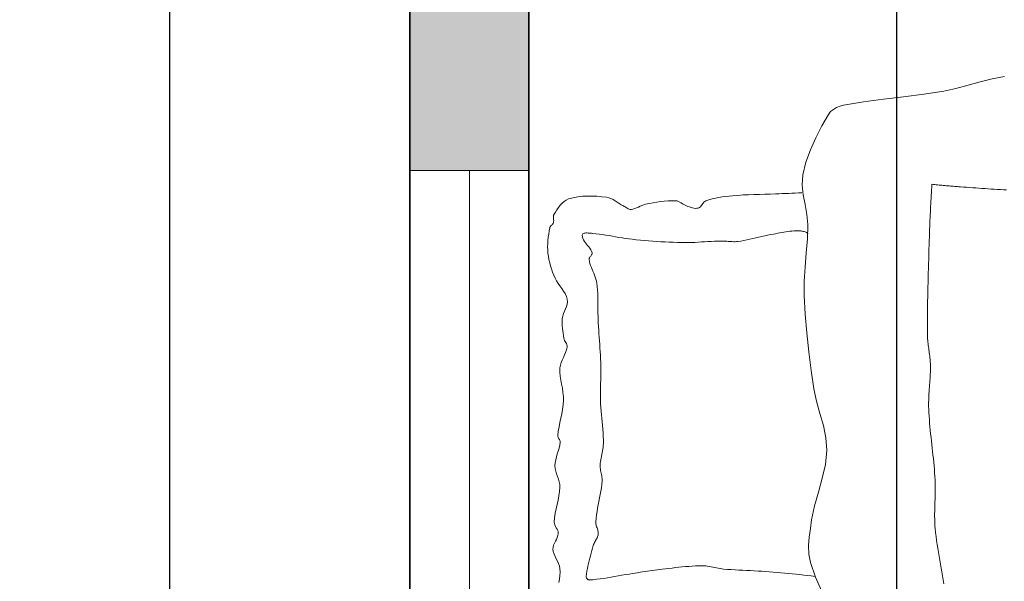
# Model space of a CAD drawing. Units: inches. Extents: x -15 to 423, y -713 to 71.
# Tile 7 of 24: x -4 to 70, y -159 to -117. Entities that reach past the tile are written whole.
import ezdxf

# ---------------------------------------------------------------- set-up
doc = ezdxf.new("R2010")
doc.units = ezdxf.units.IN
doc.header["$MEASUREMENT"] = 0
for name, color, linetype, lineweight in [('A-ANNO-DIMS', 2, 'Continuous', 18), ('A-FURN', 9, 'Continuous', 13), ('A-GLAZ', 5, 'Continuous', 18), ('A-WALL', 7, 'Continuous', 35), ('A-WALL-PATT', 8, 'Continuous', 13)]:
    doc.layers.add(name, color=color, linetype=linetype, lineweight=lineweight)
doc.styles.get("Standard").update_dxf_attribs({"font": 'arial.ttf'})
doc.dimstyles.get("Standard").update_dxf_attribs({"dimtxt": 0.18, "dimasz": 0.18, "dimexe": 0.18, "dimexo": 0.0625, "dimgap": 0.09, "dimtad": 0, "dimtih": 1, "dimtoh": 1, "dimdec": 0, "dimzin": 0, "dimdsep": 46, "dimlunit": 3, "dimtxsty": 'Standard', "dimcen": 0.09, "dimadec": 0, "dimazin": 0, "dimtfac": 1, "dimtdec": 0, "dimtofl": 0, "dimtmove": 0, "dimatfit": 3, "dimfxl": 1, "dimtolj": 1, "dimtzin": 0, "dimarcsym": 0})

# ---------------------------------------------------------------- blocks, each defined once
blk = doc.blocks.new('*D8')
at = {"layer": 'A-ANNO-DIMS', "color": 0, "lineweight": -2, "transparency": 16777216}
for p, q in [((25.018, 17.5), (6.724, 17.5)), ((6.904, 17.32), (6.904, -193.094)), ((6.904, -409.82), (6.904, -199.405)), ((34.018, -410), (6.724, -410))]:
    blk.add_line(p, q, dxfattribs=at)
at = {"layer": 'A-ANNO-DIMS', "color": 0, "transparency": 16777216}
for points in [[(6.874, 17.32), (6.934, 17.32), (6.904, 17.5)], [(6.874, -409.82), (6.934, -409.82), (6.904, -410)]]:
    blk.add_solid(points, dxfattribs=at)
at = {"layer": 'Defpoints', "color": 0, "transparency": 16777216}
for p in [(25.081, 17.5), (6.904, -410), (34.081, -410)]:
    blk.add_point(p, dxfattribs=at)
at = {"layer": 'A-ANNO-DIMS', "color": 0, "transparency": 16777216, "insert": (6.904, -196.25), "char_height": 6, "attachment_point": 5}
blk.add_mtext('\\A1;35\'-8"', dxfattribs=at)
blk = doc.blocks.new('WINDOW-60IN')
for p, q in [((0, 9), (60, 9)), ((0, 0), (0, 9)), ((60, 9), (60, 0)), ((0, 4.5), (60, 4.5)), ((60, 0), (0, 0))]:
    blk.add_line(p, q)
blk = doc.blocks.new('*D37')
at = {"layer": 'A-ANNO-DIMS', "color": 0, "lineweight": -2, "transparency": 16777216}
for p, q in [((34.081, -396.437), (34.081, 57.43)), ((61.878, -396.437), (61.878, 57.43)), ((34.261, 57.25), (47.648, 57.25)), ((61.698, 57.25), (48.31, 57.25))]:
    blk.add_line(p, q, dxfattribs=at)
at = {"layer": 'A-ANNO-DIMS', "color": 0, "transparency": 16777216}
for points in [[(34.261, 57.28), (34.261, 57.22), (34.081, 57.25)], [(61.698, 57.28), (61.698, 57.22), (61.878, 57.25)]]:
    blk.add_solid(points, dxfattribs=at)
at = {"layer": 'Defpoints', "color": 0, "transparency": 16777216}
for p in [(61.878, 57.25), (34.081, -396.5), (61.878, -396.5)]:
    blk.add_point(p, dxfattribs=at)
at = {"layer": 'A-ANNO-DIMS', "color": 0, "transparency": 16777216, "insert": (47.979, 57.25), "char_height": 0.18, "attachment_point": 5}
blk.add_mtext('\\A1;2\'-4"', dxfattribs=at)

msp = doc.modelspace()

# ---------------------------------------------------------------- hatches: boundary and pattern name
at = {"layer": 'A-WALL-PATT'}
h = msp.add_hatch(color=256, dxfattribs=at)
h.dxf.hatch_style = 1
h.paths.add_polyline_path([(34.081, -349.58), (25.081, -349.58), (25.081, -431), (34.081, -431)])
h.paths.add_polyline_path([(34.081, -467), (25.081, -467), (25.081, -673), (34.081, -673)])
h.paths.add_polyline_path([(373.081, -668.5), (182.081, -668.5), (182.081, -673), (373.081, -673)])
h.paths.add_polyline_path([(253.199, -597.5), (191.081, -597.5), (191.081, -594.5), (182.081, -594.5), (182.081, -606.5), (253.199, -606.5)])
h.paths.add_polyline_path([(373.081, -597.5), (313.199, -597.5), (313.199, -606.5), (373.081, -606.5)])
h.paths.add_polyline_path([(382.081, -545.549), (373.081, -545.549), (373.081, -673), (382.081, -673)])
h.paths.add_polyline_path([(139.081, -488), (34.081, -488), (34.081, -497), (139.081, -497), (139.081, -492.5)])
h.paths.add_polyline_path([(139.081, -396.5), (128.581, -396.5), (128.581, -352.79), (124.081, -352.79), (124.081, -396.5), (34.081, -396.5), (34.081, -410), (139.081, -410), (139.081, -403.25)])
h.paths.add_polyline_path([(191.081, -396.5), (179.081, -396.5), (179.081, -410), (182.081, -410), (182.081, -488), (179.081, -488), (179.081, -497), (182.081, -497), (182.081, -501.431), (191.081, -501.431)])
h.paths.add_polyline_path([(373.081, -396.5), (253.081, -396.5), (253.081, -393.5), (248.581, -393.5), (248.581, -401), (284.581, -401), (284.581, -404), (289.081, -404), (289.081, -401), (373.081, -401)])
h.paths.add_polyline_path([(373.081, -449), (289.081, -449), (289.081, -432), (286.831, -432), (284.581, -432), (284.581, -453.5), (373.081, -453.5)])
h.paths.add_polyline_path([(382.081, -344.267), (373.081, -344.267), (373.081, -413.683), (382.081, -413.683)])
h.paths.add_polyline_path([(382.081, -437.683), (373.081, -437.683), (373.081, -485.549), (382.081, -485.549)])
h.paths.add_polyline_path([(34.081, -188.264), (25.081, -188.264), (25.081, -289.58), (34.081, -289.58)])
h.paths.add_polyline_path([(164.081, -236), (34.081, -236), (34.081, -240.5), (124.081, -240.5), (124.081, -293.122), (128.581, -293.122), (128.581, -240.5), (164.081, -240.5), (164.081, -238.25)])
h.paths.add_polyline_path([(373.081, -236), (242.581, -236), (242.581, -238.25), (242.581, -240.5), (248.581, -240.5), (248.581, -353.5), (250.831, -353.5), (253.081, -353.5), (253.081, -240.5), (373.081, -240.5)])
h.paths.add_polyline_path([(382.081, -190.86), (373.081, -190.86), (373.081, -284.267), (382.081, -284.267)])
h.paths.add_polyline_path([(211.581, -80), (253.581, -80), (253.581, -77.75), (253.581, -75.5), (153.581, -75.5), (153.581, -77.75), (153.581, -80), (207.081, -80), (207.081, -236), (204.081, -236), (204.081, -240.5), (214.581, -240.5), (214.581, -236), (211.581, -236)])
h.paths.add_polyline_path([(34.081, 8.5), (70.358, 8.5), (70.358, 17.5), (25.081, 17.5), (25.081, -128.264), (34.081, -128.264)])
h.paths.add_polyline_path([(110.581, 17.5), (94.358, 17.5), (94.358, 8.5), (110.581, 8.5)])
h.paths.add_polyline_path([(296.581, 17.5), (110.581, 17.5), (110.581, 13), (296.581, 13)])
h.paths.add_polyline_path([(110.581, 8.5), (106.081, 8.5), (106.081, -75.5), (103.081, -75.5), (103.081, -80), (113.581, -80), (113.581, -77.75), (113.581, -75.5), (110.581, -75.5)])
h.paths.add_polyline_path([(75.081, -75.5), (34.081, -75.5), (34.081, -80), (75.081, -80), (75.081, -77.75)])
h.paths.add_polyline_path([(343.093, 17.5), (296.581, 17.5), (296.581, 13), (296.581, 8.5), (343.093, 8.5)])
h.paths.add_polyline_path([(304.081, -75.5), (301.081, -75.5), (301.081, 8.5), (296.581, 8.5), (296.581, -75.5), (293.581, -75.5), (293.581, -80), (304.081, -80)])
h.paths.add_polyline_path([(382.081, 17.5), (367.093, 17.5), (367.093, 8.5), (373.081, 8.5), (373.081, -130.86), (382.081, -130.86)])
h.paths.add_polyline_path([(373.081, -75.5), (332.081, -75.5), (332.081, -77.75), (332.081, -80), (373.081, -80)])

# ---------------------------------------------------------------- linework, layer by layer
at = {"layer": 'A-FURN'}
for p, q in [((70.017, -121.158), (69.09, -121.325)), ((67.264, -121.811), (66.352, -122.057)), ((68.175, -121.555), (67.264, -121.811)), ((69.09, -121.325), (68.175, -121.555)), ((62.4, -122.683), (60.879, -122.863)), ((63.919, -122.493), (62.4, -122.683)), ((65.43, -122.258), (63.919, -122.493)), ((66.352, -122.057), (65.43, -122.258)), ((57.333, -123.497), (57.091, -123.633)), ((57.593, -123.396), (57.333, -123.497)), ((57.856, -123.328), (57.593, -123.396)), ((59.363, -123.066), (57.856, -123.328)), ((60.879, -122.863), (59.363, -123.066)), ((56.72, -124.015), (56.225, -124.884)), ((56.882, -123.805), (56.72, -124.015)), ((57.091, -123.633), (56.882, -123.805)), ((56.225, -124.884), (55.76, -125.775)), ((55.76, -125.775), (55.349, -126.69)), ((55.349, -126.69), (55.012, -127.629)), ((55.012, -127.629), (54.771, -128.593)), ((54.771, -128.593), (54.72, -129.335)), ((54.72, -129.335), (54.801, -130.081)), ((64.541, -129.293), (64.527, -129.504)), ((64.648, -129.305), (64.541, -129.293)), ((64.755, -129.317), (64.648, -129.305)), ((64.862, -129.328), (64.755, -129.317)), ((64.969, -129.34), (64.862, -129.328)), ((65.076, -129.351), (64.969, -129.34)), ((65.184, -129.362), (65.076, -129.351)), ((65.291, -129.373), (65.184, -129.362)), ((65.398, -129.383), (65.291, -129.373)), ((65.506, -129.393), (65.398, -129.383)), ((65.613, -129.403), (65.506, -129.393)), ((65.72, -129.413), (65.613, -129.403)), ((65.828, -129.422), (65.72, -129.413)), ((65.935, -129.431), (65.828, -129.422)), ((66.043, -129.44), (65.935, -129.431)), ((66.15, -129.448), (66.043, -129.44)), ((66.257, -129.457), (66.15, -129.448)), ((66.365, -129.465), (66.257, -129.457)), ((66.472, -129.473), (66.365, -129.465)), ((66.58, -129.48), (66.472, -129.473)), ((66.687, -129.487), (66.58, -129.48)), ((38.136, -130.201), (37.779, -130.242)), ((38.497, -130.183), (38.136, -130.201)), ((38.86, -130.184), (38.497, -130.183)), ((39.223, -130.202), (38.86, -130.184)), ((39.584, -130.232), (39.223, -130.202)), ((48.945, -130.219), (48.69, -130.253)), ((49.2, -130.19), (48.945, -130.219)), ((49.455, -130.164), (49.2, -130.19)), ((49.862, -130.13), (49.455, -130.164)), ((50.271, -130.104), (49.862, -130.13)), ((50.68, -130.085), (50.271, -130.104)), ((51.089, -130.072), (50.68, -130.085)), ((51.498, -130.061), (51.089, -130.072)), ((51.908, -130.05), (51.498, -130.061)), ((52.317, -130.038), (51.908, -130.05)), ((52.726, -130.023), (52.317, -130.038)), ((52.973, -130.012), (52.726, -130.023)), ((53.22, -130.001), (52.973, -130.012)), ((53.467, -129.99), (53.22, -130.001)), ((53.714, -129.979), (53.467, -129.99)), ((53.961, -129.968), (53.714, -129.979)), ((54.207, -129.957), (53.961, -129.968)), ((54.454, -129.945), (54.207, -129.957)), ((54.701, -129.934), (54.454, -129.945)), ((54.801, -130.081), (54.945, -130.83)), ((64.487, -130.137), (64.475, -130.349)), ((64.5, -129.926), (64.487, -130.137)), ((64.513, -129.715), (64.5, -129.926)), ((64.527, -129.504), (64.513, -129.715)), ((66.92, -129.503), (66.687, -129.487)), ((67.153, -129.52), (66.92, -129.503)), ((67.386, -129.537), (67.153, -129.52)), ((67.619, -129.555), (67.386, -129.537)), ((67.852, -129.572), (67.619, -129.555)), ((68.085, -129.59), (67.852, -129.572)), ((68.318, -129.608), (68.085, -129.59)), ((68.551, -129.625), (68.318, -129.608)), ((68.784, -129.642), (68.551, -129.625)), ((69.017, -129.658), (68.784, -129.642)), ((69.25, -129.674), (69.017, -129.658)), ((69.483, -129.688), (69.25, -129.674)), ((69.716, -129.701), (69.483, -129.688)), ((69.949, -129.713), (69.716, -129.701)), ((70.182, -129.723), (69.949, -129.713)), ((36.448, -130.877), (36.32, -131.043)), ((36.586, -130.725), (36.448, -130.877)), ((36.736, -130.592), (36.586, -130.725)), ((36.901, -130.483), (36.736, -130.592)), ((37.082, -130.404), (36.901, -130.483)), ((37.427, -130.309), (37.082, -130.404)), ((37.779, -130.242), (37.427, -130.309)), ((39.942, -130.273), (39.584, -130.232)), ((40.115, -130.309), (39.942, -130.273)), ((40.28, -130.369), (40.115, -130.309)), ((40.44, -130.448), (40.28, -130.369)), ((40.595, -130.54), (40.44, -130.448)), ((40.749, -130.638), (40.595, -130.54)), ((40.902, -130.739), (40.749, -130.638)), ((41.057, -130.835), (40.902, -130.739)), ((41.214, -130.921), (41.057, -130.835)), ((41.286, -130.961), (41.214, -130.921)), ((41.356, -131.007), (41.286, -130.961)), ((42.485, -130.949), (42.351, -131.014)), ((42.621, -130.888), (42.485, -130.949)), ((42.759, -130.835), (42.621, -130.888)), ((42.9, -130.798), (42.759, -130.835)), ((43.18, -130.743), (42.9, -130.798)), ((43.46, -130.691), (43.18, -130.743)), ((43.742, -130.643), (43.46, -130.691)), ((44.025, -130.601), (43.742, -130.643)), ((44.308, -130.567), (44.025, -130.601)), ((44.591, -130.544), (44.308, -130.567)), ((44.875, -130.533), (44.591, -130.544)), ((45.159, -130.537), (44.875, -130.533)), ((45.271, -130.554), (45.159, -130.537)), ((45.378, -130.59), (45.271, -130.554)), ((45.481, -130.642), (45.378, -130.59)), ((45.581, -130.702), (45.481, -130.642)), ((45.681, -130.767), (45.581, -130.702)), ((45.782, -130.829), (45.681, -130.767)), ((45.886, -130.885), (45.782, -130.829)), ((45.993, -130.928), (45.886, -130.885)), ((46.101, -130.965), (45.993, -130.928)), ((46.212, -131.004), (46.101, -130.965)), ((47.107, -130.912), (47.042, -130.99)), ((47.166, -130.826), (47.107, -130.912)), ((47.226, -130.738), (47.166, -130.826)), ((47.289, -130.657), (47.226, -130.738)), ((47.361, -130.589), (47.289, -130.657)), ((47.446, -130.543), (47.361, -130.589)), ((47.688, -130.463), (47.446, -130.543)), ((47.935, -130.396), (47.688, -130.463)), ((48.184, -130.339), (47.935, -130.396)), ((48.436, -130.292), (48.184, -130.339)), ((48.69, -130.253), (48.436, -130.292)), ((54.945, -130.83), (55.084, -131.581)), ((64.451, -130.771), (64.44, -130.982)), ((64.462, -130.56), (64.451, -130.771)), ((64.475, -130.349), (64.462, -130.56)), ((35.931, -131.711), (35.93, -131.791)), ((35.945, -131.634), (35.931, -131.711)), ((35.978, -131.564), (35.945, -131.634)), ((36.087, -131.391), (35.978, -131.564)), ((36.2, -131.216), (36.087, -131.391)), ((36.32, -131.043), (36.2, -131.216)), ((41.427, -131.054), (41.356, -131.007)), ((41.498, -131.1), (41.427, -131.054)), ((41.57, -131.141), (41.498, -131.1)), ((41.643, -131.173), (41.57, -131.141)), ((41.719, -131.192), (41.643, -131.173)), ((41.798, -131.195), (41.719, -131.192)), ((41.941, -131.173), (41.798, -131.195)), ((42.08, -131.132), (41.941, -131.173)), ((42.216, -131.077), (42.08, -131.132)), ((42.351, -131.014), (42.216, -131.077)), ((46.323, -131.041), (46.212, -131.004)), ((46.436, -131.074), (46.323, -131.041)), ((46.548, -131.099), (46.436, -131.074)), ((46.661, -131.112), (46.548, -131.099)), ((46.772, -131.111), (46.661, -131.112)), ((46.882, -131.092), (46.772, -131.111)), ((46.969, -131.053), (46.882, -131.092)), ((47.042, -130.99), (46.969, -131.053)), ((55.084, -131.581), (55.151, -132.332)), ((64.408, -131.617), (64.398, -131.828)), ((64.418, -131.405), (64.408, -131.617)), ((64.429, -131.194), (64.418, -131.405)), ((64.44, -130.982), (64.429, -131.194)), ((35.74, -132.433), (35.701, -132.478)), ((35.785, -132.39), (35.74, -132.433)), ((35.83, -132.348), (35.785, -132.39)), ((35.872, -132.303), (35.83, -132.348)), ((35.907, -132.256), (35.872, -132.303)), ((35.932, -132.203), (35.907, -132.256)), ((35.93, -131.791), (35.936, -131.875)), ((35.948, -132.125), (35.932, -132.203)), ((35.936, -131.875), (35.944, -131.959)), ((35.944, -131.959), (35.95, -132.043)), ((35.95, -132.043), (35.948, -132.125)), ((55.151, -132.332), (55.123, -133.406)), ((64.38, -132.251), (64.372, -132.462)), ((64.389, -132.039), (64.38, -132.251)), ((64.398, -131.828), (64.389, -132.039)), ((35.573, -133.057), (35.54, -133.297)), ((35.611, -132.818), (35.573, -133.057)), ((35.652, -132.581), (35.611, -132.818)), ((35.67, -132.526), (35.652, -132.581)), ((35.701, -132.478), (35.67, -132.526)), ((38.107, -133.149), (38.118, -133.09)), ((38.117, -133.272), (38.107, -133.149)), ((38.118, -133.09), (38.148, -133.045)), ((38.148, -133.045), (38.194, -133.013)), ((38.194, -133.013), (38.253, -132.99)), ((38.253, -132.99), (38.322, -132.977)), ((38.322, -132.977), (38.4, -132.971)), ((38.4, -132.971), (38.482, -132.971)), ((38.482, -132.971), (38.568, -132.976)), ((38.568, -132.976), (38.654, -132.983)), ((38.654, -132.983), (38.737, -132.992)), ((38.737, -132.992), (38.816, -133)), ((38.816, -133), (38.886, -133.007)), ((38.886, -133.007), (39.137, -133.03)), ((39.137, -133.03), (39.388, -133.06)), ((39.388, -133.06), (39.638, -133.095)), ((39.638, -133.095), (39.887, -133.134)), ((39.887, -133.134), (40.136, -133.175)), ((40.136, -133.175), (40.385, -133.219)), ((51.672, -133.244), (51.897, -133.193)), ((51.897, -133.193), (52.122, -133.143)), ((52.122, -133.143), (52.347, -133.097)), ((52.347, -133.097), (52.573, -133.054)), ((52.573, -133.054), (52.726, -133.027)), ((52.726, -133.027), (52.879, -132.999)), ((52.879, -132.999), (53.033, -132.971)), ((53.033, -132.971), (53.186, -132.943)), ((53.186, -132.943), (53.34, -132.917)), ((53.34, -132.917), (53.494, -132.892)), ((53.494, -132.892), (53.647, -132.869)), ((53.647, -132.869), (53.802, -132.849)), ((53.802, -132.849), (53.956, -132.832)), ((53.956, -132.832), (54.111, -132.818)), ((54.111, -132.818), (54.266, -132.808)), ((54.266, -132.808), (54.421, -132.803)), ((54.421, -132.803), (54.487, -132.804)), ((54.487, -132.804), (54.554, -132.808)), ((54.554, -132.808), (54.621, -132.815)), ((54.621, -132.815), (54.687, -132.825)), ((54.687, -132.825), (54.753, -132.838)), ((54.753, -132.838), (54.819, -132.854)), ((54.819, -132.854), (54.884, -132.873)), ((54.884, -132.873), (54.947, -132.895)), ((54.947, -132.895), (55.01, -132.92)), ((55.01, -132.92), (55.071, -132.948)), ((55.071, -132.948), (55.13, -132.978)), ((55.13, -132.978), (55.188, -133.011)), ((64.348, -133.097), (64.341, -133.308)), ((64.356, -132.885), (64.348, -133.097)), ((64.363, -132.674), (64.356, -132.885)), ((64.372, -132.462), (64.363, -132.674)), ((35.498, -133.779), (35.491, -134.019)), ((35.515, -133.538), (35.498, -133.779)), ((35.54, -133.297), (35.515, -133.538)), ((38.15, -133.389), (38.117, -133.272)), ((38.201, -133.501), (38.15, -133.389)), ((38.267, -133.608), (38.201, -133.501)), ((38.344, -133.713), (38.267, -133.608)), ((38.428, -133.817), (38.344, -133.713)), ((38.515, -133.92), (38.428, -133.817)), ((38.601, -134.023), (38.515, -133.92)), ((40.385, -133.219), (40.634, -133.263)), ((40.634, -133.263), (40.883, -133.306)), ((40.883, -133.306), (41.133, -133.347)), ((41.133, -133.347), (41.382, -133.385)), ((41.382, -133.385), (41.633, -133.42)), ((41.633, -133.42), (41.883, -133.448)), ((41.883, -133.448), (42.193, -133.48)), ((42.193, -133.48), (42.502, -133.509)), ((42.502, -133.509), (42.812, -133.538)), ((42.812, -133.538), (43.122, -133.564)), ((43.122, -133.564), (43.432, -133.589)), ((43.432, -133.589), (43.743, -133.611)), ((43.743, -133.611), (44.053, -133.632)), ((44.053, -133.632), (44.364, -133.65)), ((44.364, -133.65), (44.674, -133.666)), ((44.674, -133.666), (44.985, -133.679)), ((44.985, -133.679), (45.296, -133.69)), ((45.296, -133.69), (45.607, -133.698)), ((45.607, -133.698), (45.857, -133.7)), ((45.857, -133.7), (46.108, -133.698)), ((46.108, -133.698), (46.358, -133.691)), ((46.358, -133.691), (46.608, -133.681)), ((46.608, -133.681), (46.859, -133.669)), ((46.859, -133.669), (47.109, -133.655)), ((47.109, -133.655), (47.359, -133.641)), ((47.359, -133.641), (47.61, -133.626)), ((47.61, -133.626), (47.86, -133.612)), ((47.86, -133.612), (48.11, -133.6)), ((48.11, -133.6), (48.361, -133.59)), ((48.361, -133.59), (48.611, -133.583)), ((48.611, -133.583), (48.716, -133.583)), ((48.716, -133.583), (48.821, -133.587)), ((48.821, -133.587), (48.926, -133.593)), ((48.926, -133.593), (49.031, -133.6)), ((49.031, -133.6), (49.136, -133.608)), ((49.136, -133.608), (49.241, -133.617)), ((49.241, -133.617), (49.346, -133.624)), ((49.346, -133.624), (49.451, -133.629)), ((49.451, -133.629), (49.555, -133.632)), ((49.555, -133.632), (49.66, -133.631)), ((49.66, -133.631), (49.764, -133.625)), ((49.764, -133.625), (49.868, -133.615)), ((49.868, -133.615), (50.096, -133.581)), ((50.096, -133.581), (50.323, -133.542)), ((50.323, -133.542), (50.548, -133.498)), ((50.548, -133.498), (50.774, -133.451)), ((50.774, -133.451), (50.999, -133.401)), ((50.999, -133.401), (51.223, -133.349)), ((51.223, -133.349), (51.448, -133.297)), ((51.448, -133.297), (51.672, -133.244)), ((55.123, -133.406), (55.041, -134.478)), ((64.324, -133.875), (64.313, -134.23)), ((64.335, -133.52), (64.324, -133.875)), ((64.341, -133.308), (64.335, -133.52)), ((35.491, -134.019), (35.496, -134.26)), ((35.496, -134.26), (35.514, -134.5)), ((35.514, -134.5), (35.546, -134.742)), ((38.682, -134.129), (38.601, -134.023)), ((38.755, -134.238), (38.682, -134.129)), ((38.751, -134.718), (38.785, -134.678)), ((38.816, -134.351), (38.755, -134.238)), ((38.785, -134.678), (38.815, -134.637)), ((38.815, -134.637), (38.841, -134.597)), ((38.86, -134.47), (38.816, -134.351)), ((38.841, -134.597), (38.858, -134.555)), ((38.858, -134.555), (38.865, -134.513)), ((38.865, -134.513), (38.86, -134.47)), ((55.041, -134.478), (54.945, -135.55)), ((64.302, -134.586), (64.291, -134.941)), ((64.313, -134.23), (64.302, -134.586)), ((35.546, -134.742), (35.592, -134.983)), ((35.592, -134.983), (35.648, -135.222)), ((35.648, -135.222), (35.715, -135.458)), ((38.625, -134.925), (38.636, -134.882)), ((38.625, -134.97), (38.625, -134.925)), ((38.654, -135.124), (38.625, -134.97)), ((38.636, -134.882), (38.657, -134.84)), ((38.694, -135.276), (38.654, -135.124)), ((38.657, -134.84), (38.685, -134.798)), ((38.685, -134.798), (38.717, -134.758)), ((38.742, -135.426), (38.694, -135.276)), ((38.717, -134.758), (38.751, -134.718)), ((38.797, -135.574), (38.742, -135.426)), ((64.28, -135.297), (64.27, -135.652)), ((64.291, -134.941), (64.28, -135.297)), ((35.715, -135.458), (35.79, -135.693)), ((35.79, -135.693), (35.872, -135.925)), ((35.872, -135.925), (35.961, -136.154)), ((35.961, -136.154), (36.054, -136.381)), ((38.855, -135.722), (38.797, -135.574)), ((38.916, -135.869), (38.855, -135.722)), ((38.976, -136.016), (38.916, -135.869)), ((39.035, -136.163), (38.976, -136.016)), ((39.089, -136.312), (39.035, -136.163)), ((54.945, -135.55), (54.875, -136.622)), ((64.26, -136.008), (64.25, -136.363)), ((64.27, -135.652), (64.26, -136.008)), ((36.054, -136.381), (36.158, -136.589)), ((36.158, -136.589), (36.284, -136.787)), ((36.284, -136.787), (36.423, -136.979)), ((39.137, -136.462), (39.089, -136.312)), ((39.176, -136.614), (39.137, -136.462)), ((39.204, -136.768), (39.176, -136.614)), ((39.236, -137.016), (39.204, -136.768)), ((54.875, -136.622), (54.87, -137.694)), ((64.241, -136.718), (64.232, -137.074)), ((64.25, -136.363), (64.241, -136.718)), ((36.423, -136.979), (36.565, -137.169)), ((36.565, -137.169), (36.701, -137.361)), ((36.701, -137.361), (36.822, -137.559)), ((36.822, -137.559), (36.917, -137.766)), ((39.259, -137.265), (39.236, -137.016)), ((39.275, -137.515), (39.259, -137.265)), ((39.286, -137.765), (39.275, -137.515)), ((64.224, -137.429), (64.217, -137.785)), ((64.232, -137.074), (64.224, -137.429)), ((36.963, -138.35), (36.91, -138.53)), ((36.917, -137.766), (36.979, -137.986)), ((36.99, -138.169), (36.963, -138.35)), ((36.979, -137.986), (36.99, -138.169)), ((39.293, -138.016), (39.286, -137.765)), ((39.296, -138.267), (39.293, -138.016)), ((39.297, -138.518), (39.296, -138.267)), ((54.87, -137.694), (54.948, -139.113)), ((64.211, -138.14), (64.205, -138.496)), ((64.217, -137.785), (64.211, -138.14)), ((36.692, -139.069), (36.634, -139.252)), ((36.764, -138.889), (36.692, -139.069)), ((36.84, -138.709), (36.764, -138.889)), ((36.91, -138.53), (36.84, -138.709)), ((39.298, -138.769), (39.297, -138.518)), ((39.299, -139.02), (39.298, -138.769)), ((39.302, -139.271), (39.299, -139.02)), ((54.948, -139.113), (55.072, -140.53)), ((64.201, -138.851), (64.198, -139.207)), ((64.205, -138.496), (64.201, -138.851)), ((36.602, -139.437), (36.591, -139.622)), ((36.591, -139.622), (36.591, -139.807)), ((36.591, -139.807), (36.599, -139.993)), ((36.634, -139.252), (36.602, -139.437)), ((39.308, -139.522), (39.302, -139.271)), ((39.319, -139.772), (39.308, -139.522)), ((39.333, -140.043), (39.319, -139.772)), ((64.198, -139.207), (64.196, -139.562)), ((64.196, -139.562), (64.196, -139.918)), ((36.599, -139.993), (36.614, -140.179)), ((36.614, -140.179), (36.636, -140.364)), ((36.636, -140.364), (36.661, -140.549)), ((36.661, -140.549), (36.69, -140.733)), ((39.351, -140.314), (39.333, -140.043)), ((39.369, -140.585), (39.351, -140.314)), ((39.389, -140.855), (39.369, -140.585)), ((55.072, -140.53), (55.231, -141.943)), ((64.196, -139.918), (64.196, -140.273)), ((64.196, -140.273), (64.199, -140.629)), ((64.199, -140.629), (64.201, -140.746)), ((36.69, -140.733), (36.72, -140.917)), ((36.72, -140.917), (36.743, -141.004)), ((36.743, -141.004), (36.779, -141.088)), ((36.779, -141.088), (36.823, -141.171)), ((36.823, -141.171), (36.868, -141.253)), ((36.868, -141.253), (36.911, -141.335)), ((36.911, -141.335), (36.944, -141.419)), ((39.409, -141.126), (39.389, -140.855)), ((39.429, -141.396), (39.409, -141.126)), ((64.201, -140.746), (64.206, -140.864)), ((64.206, -140.864), (64.214, -140.981)), ((64.214, -140.981), (64.223, -141.098)), ((64.223, -141.098), (64.235, -141.215)), ((64.235, -141.215), (64.247, -141.332)), ((64.247, -141.332), (64.261, -141.449)), ((36.854, -141.992), (36.771, -142.186)), ((36.921, -141.794), (36.854, -141.992)), ((36.963, -141.591), (36.921, -141.794)), ((36.944, -141.419), (36.963, -141.503)), ((36.963, -141.503), (36.963, -141.591)), ((39.449, -141.667), (39.429, -141.396)), ((39.467, -141.938), (39.449, -141.667)), ((39.485, -142.209), (39.467, -141.938)), ((55.231, -141.943), (55.416, -143.354)), ((64.261, -141.449), (64.276, -141.566)), ((64.276, -141.566), (64.292, -141.683)), ((64.292, -141.683), (64.307, -141.8)), ((64.307, -141.8), (64.323, -141.917)), ((64.323, -141.917), (64.339, -142.034)), ((64.339, -142.034), (64.354, -142.151)), ((36.515, -142.766), (36.456, -142.965)), ((36.593, -142.571), (36.515, -142.766)), ((36.681, -142.378), (36.593, -142.571)), ((36.771, -142.186), (36.681, -142.378)), ((39.5, -142.479), (39.485, -142.209)), ((39.512, -142.75), (39.5, -142.479)), ((39.521, -143.021), (39.512, -142.75)), ((64.354, -142.151), (64.368, -142.268)), ((64.368, -142.268), (64.381, -142.385)), ((64.381, -142.385), (64.393, -142.502)), ((64.393, -142.502), (64.403, -142.619)), ((64.403, -142.619), (64.411, -142.736)), ((64.411, -142.736), (64.417, -142.854)), ((64.417, -142.854), (64.421, -142.971)), ((36.425, -143.169), (36.422, -143.478)), ((36.422, -143.478), (36.447, -143.786)), ((36.456, -142.965), (36.425, -143.169)), ((39.525, -143.236), (39.521, -143.021)), ((39.521, -143.665), (39.525, -143.451)), ((39.525, -143.451), (39.525, -143.236)), ((55.416, -143.354), (55.618, -144.761)), ((64.417, -143.466), (64.411, -143.631)), ((64.42, -143.301), (64.417, -143.466)), ((64.422, -143.136), (64.42, -143.301)), ((64.421, -142.971), (64.422, -143.136)), ((36.447, -143.786), (36.492, -144.093)), ((36.492, -144.093), (36.547, -144.401)), ((39.492, -144.524), (39.5, -144.309)), ((39.5, -144.309), (39.508, -144.095)), ((39.508, -144.095), (39.515, -143.88)), ((39.515, -143.88), (39.521, -143.665)), ((64.372, -144.291), (64.36, -144.456)), ((64.383, -144.126), (64.372, -144.291)), ((64.393, -143.961), (64.383, -144.126)), ((64.403, -143.796), (64.393, -143.961)), ((64.411, -143.631), (64.403, -143.796)), ((36.547, -144.401), (36.604, -144.708)), ((36.604, -144.708), (36.653, -145.016)), ((36.653, -145.016), (36.685, -145.325)), ((39.476, -145.168), (39.479, -144.953)), ((39.479, -144.953), (39.485, -144.739)), ((39.485, -144.739), (39.492, -144.524)), ((55.618, -144.761), (55.811, -145.691)), ((64.325, -144.951), (64.315, -145.115)), ((64.336, -144.786), (64.325, -144.951)), ((64.348, -144.621), (64.336, -144.786)), ((64.36, -144.456), (64.348, -144.621)), ((36.691, -145.634), (36.667, -145.968)), ((36.685, -145.325), (36.691, -145.634)), ((39.477, -145.382), (39.476, -145.168)), ((39.481, -145.597), (39.477, -145.382)), ((39.493, -145.873), (39.481, -145.597)), ((55.811, -145.691), (56.07, -146.611)), ((64.289, -145.775), (64.288, -145.94)), ((64.293, -145.61), (64.289, -145.775)), ((64.298, -145.445), (64.293, -145.61)), ((64.306, -145.28), (64.298, -145.445)), ((64.315, -145.115), (64.306, -145.28)), ((36.622, -146.299), (36.561, -146.629)), ((36.667, -145.968), (36.622, -146.299)), ((39.51, -146.149), (39.493, -145.873)), ((39.531, -146.425), (39.51, -146.149)), ((39.556, -146.701), (39.531, -146.425)), ((64.288, -145.94), (64.29, -146.105)), ((64.29, -146.105), (64.295, -146.27)), ((64.295, -146.27), (64.308, -146.539)), ((64.308, -146.539), (64.324, -146.807)), ((36.421, -147.287), (36.355, -147.617)), ((36.492, -146.958), (36.421, -147.287)), ((36.561, -146.629), (36.492, -146.958)), ((39.582, -146.976), (39.556, -146.701)), ((39.608, -147.252), (39.582, -146.976)), ((39.634, -147.528), (39.608, -147.252)), ((56.07, -146.611), (56.33, -147.53)), ((64.324, -146.807), (64.343, -147.076)), ((64.343, -147.076), (64.364, -147.344)), ((36.299, -147.948), (36.261, -148.281)), ((36.355, -147.617), (36.299, -147.948)), ((39.658, -147.803), (39.634, -147.528)), ((39.678, -148.079), (39.658, -147.803)), ((39.693, -148.355), (39.678, -148.079)), ((56.33, -147.53), (56.527, -148.455)), ((64.364, -147.344), (64.388, -147.612)), ((64.388, -147.612), (64.413, -147.88)), ((64.413, -147.88), (64.44, -148.148)), ((36.261, -148.281), (36.265, -148.344)), ((36.265, -148.344), (36.285, -148.406)), ((36.285, -148.406), (36.315, -148.466)), ((36.315, -148.466), (36.35, -148.526)), ((36.35, -148.526), (36.385, -148.585)), ((36.385, -148.585), (36.415, -148.646)), ((36.438, -148.771), (36.405, -148.999)), ((36.415, -148.646), (36.434, -148.707)), ((36.434, -148.707), (36.438, -148.771)), ((39.703, -148.631), (39.693, -148.355)), ((39.706, -148.907), (39.703, -148.631)), ((56.527, -148.455), (56.596, -149.392)), ((64.44, -148.148), (64.468, -148.416)), ((64.468, -148.416), (64.497, -148.684)), ((64.497, -148.684), (64.527, -148.952)), ((36.291, -149.448), (36.224, -149.67)), ((36.354, -149.224), (36.291, -149.448)), ((36.405, -148.999), (36.354, -149.224)), ((39.617, -149.58), (39.644, -149.446)), ((39.644, -149.446), (39.668, -149.312)), ((39.668, -149.312), (39.688, -149.178)), ((39.688, -149.178), (39.701, -149.043)), ((39.701, -149.043), (39.706, -148.907)), ((56.596, -149.392), (56.489, -150.458)), ((64.527, -148.952), (64.556, -149.22)), ((64.556, -149.22), (64.586, -149.488)), ((64.586, -149.488), (64.615, -149.756)), ((36.104, -150.117), (36.065, -150.343)), ((36.159, -149.893), (36.104, -150.117)), ((36.224, -149.67), (36.159, -149.893)), ((39.465, -150.384), (39.481, -150.25)), ((39.481, -150.25), (39.503, -150.115)), ((39.503, -150.115), (39.529, -149.981)), ((39.529, -149.981), (39.558, -149.847)), ((39.558, -149.847), (39.587, -149.714)), ((39.587, -149.714), (39.617, -149.58)), ((64.615, -149.756), (64.643, -150.023)), ((64.643, -150.023), (64.67, -150.291)), ((64.67, -150.291), (64.696, -150.56)), ((36.065, -150.343), (36.049, -150.572)), ((36.049, -150.572), (36.064, -150.775)), ((36.064, -150.775), (36.107, -150.975)), ((36.107, -150.975), (36.167, -151.174)), ((39.457, -150.52), (39.465, -150.384)), ((39.457, -150.62), (39.457, -150.52)), ((39.465, -150.719), (39.457, -150.62)), ((39.479, -150.819), (39.465, -150.719)), ((39.497, -150.918), (39.479, -150.819)), ((39.518, -151.017), (39.497, -150.918)), ((39.539, -151.116), (39.518, -151.017)), ((56.489, -150.458), (56.253, -151.507)), ((64.696, -150.56), (64.719, -150.828)), ((64.719, -150.828), (64.741, -151.096)), ((36.167, -151.174), (36.235, -151.371)), ((36.235, -151.371), (36.304, -151.568)), ((36.304, -151.568), (36.363, -151.766)), ((36.363, -151.766), (36.404, -151.966)), ((39.561, -151.215), (39.539, -151.116)), ((39.58, -151.314), (39.561, -151.215)), ((39.596, -151.413), (39.58, -151.314)), ((39.585, -151.969), (39.609, -151.711)), ((39.608, -151.512), (39.596, -151.413)), ((39.612, -151.611), (39.608, -151.512)), ((39.609, -151.711), (39.612, -151.611)), ((56.253, -151.507), (55.954, -152.55)), ((64.741, -151.096), (64.76, -151.365)), ((64.76, -151.365), (64.776, -151.634)), ((64.776, -151.634), (64.784, -151.817)), ((36.397, -152.503), (36.349, -152.835)), ((36.418, -152.17), (36.397, -152.503)), ((36.404, -151.966), (36.418, -152.17)), ((39.466, -152.74), (39.511, -152.484)), ((39.511, -152.484), (39.551, -152.227)), ((39.551, -152.227), (39.585, -151.969)), ((55.954, -152.55), (55.663, -153.595)), ((64.784, -151.817), (64.789, -152)), ((64.788, -152.55), (64.785, -152.734)), ((64.791, -152.367), (64.788, -152.55)), ((64.789, -152), (64.791, -152.183)), ((64.791, -152.183), (64.791, -152.367)), ((36.284, -153.164), (36.209, -153.493)), ((36.349, -152.835), (36.284, -153.164)), ((39.318, -153.507), (39.368, -153.251)), ((39.368, -153.251), (39.418, -152.995)), ((39.418, -152.995), (39.466, -152.74)), ((64.767, -153.284), (64.761, -153.468)), ((64.773, -153.101), (64.767, -153.284)), ((64.779, -152.917), (64.773, -153.101)), ((64.785, -152.734), (64.779, -152.917)), ((36.134, -153.822), (36.066, -154.152)), ((36.209, -153.493), (36.134, -153.822)), ((39.185, -154.275), (39.224, -154.019)), ((39.224, -154.019), (39.269, -153.762)), ((39.269, -153.762), (39.318, -153.507)), ((55.663, -153.595), (55.447, -154.651)), ((64.745, -154.018), (64.743, -154.202)), ((64.749, -153.835), (64.745, -154.018)), ((64.755, -153.651), (64.749, -153.835)), ((64.761, -153.468), (64.755, -153.651)), ((36.015, -154.483), (35.988, -154.816)), ((36.066, -154.152), (36.015, -154.483)), ((39.128, -154.791), (39.152, -154.533)), ((39.152, -154.533), (39.185, -154.275)), ((55.447, -154.651), (55.35, -155.295)), ((64.743, -154.202), (64.742, -154.385)), ((64.742, -154.385), (64.744, -154.568)), ((64.744, -154.568), (64.749, -154.751)), ((64.749, -154.751), (64.756, -154.934)), ((35.988, -154.816), (35.999, -154.928)), ((35.999, -154.928), (36.034, -155.036)), ((36.034, -155.036), (36.085, -155.141)), ((36.085, -155.141), (36.144, -155.245)), ((36.144, -155.245), (36.203, -155.349)), ((36.203, -155.349), (36.253, -155.455)), ((36.253, -155.455), (36.287, -155.562)), ((39.128, -154.868), (39.128, -154.791)), ((39.136, -154.943), (39.128, -154.868)), ((39.152, -155.018), (39.136, -154.943)), ((39.173, -155.093), (39.152, -155.018)), ((39.198, -155.168), (39.173, -155.093)), ((39.225, -155.242), (39.198, -155.168)), ((39.251, -155.317), (39.225, -155.242)), ((39.275, -155.392), (39.251, -155.317)), ((39.296, -155.466), (39.275, -155.392)), ((39.31, -155.541), (39.296, -155.466)), ((55.35, -155.295), (55.262, -155.945)), ((64.756, -154.934), (64.767, -155.117)), ((64.767, -155.117), (64.783, -155.3)), ((64.783, -155.3), (64.814, -155.6)), ((36.081, -156.266), (36.007, -156.41)), ((36.156, -156.122), (36.081, -156.266)), ((36.223, -155.976), (36.156, -156.122)), ((36.273, -155.827), (36.223, -155.976)), ((36.297, -155.674), (36.273, -155.827)), ((36.287, -155.562), (36.297, -155.674)), ((39.073, -156.289), (39.112, -156.217)), ((39.112, -156.217), (39.151, -156.144)), ((39.151, -156.144), (39.189, -156.072)), ((39.189, -156.072), (39.224, -155.999)), ((39.224, -155.999), (39.256, -155.925)), ((39.256, -155.925), (39.282, -155.849)), ((39.282, -155.849), (39.302, -155.772)), ((39.302, -155.772), (39.315, -155.693)), ((39.317, -155.617), (39.31, -155.541)), ((39.315, -155.693), (39.317, -155.617)), ((55.262, -155.945), (55.215, -156.596)), ((64.814, -155.6), (64.849, -155.9)), ((64.849, -155.9), (64.888, -156.199)), ((64.888, -156.199), (64.931, -156.498)), ((35.904, -156.704), (35.893, -156.858)), ((35.893, -156.858), (35.92, -157.049)), ((35.945, -156.556), (35.904, -156.704)), ((36.007, -156.41), (35.945, -156.556)), ((38.783, -157.167), (38.837, -156.973)), ((38.837, -156.973), (38.891, -156.78)), ((38.891, -156.78), (38.945, -156.588)), ((38.945, -156.588), (38.97, -156.511)), ((38.97, -156.511), (39.001, -156.436)), ((39.001, -156.436), (39.035, -156.362)), ((39.035, -156.362), (39.073, -156.289)), ((55.215, -156.596), (55.238, -157.239)), ((64.931, -156.498), (64.976, -156.796)), ((64.976, -156.796), (65.024, -157.095)), ((35.92, -157.049), (35.977, -157.234)), ((35.977, -157.234), (36.053, -157.415)), ((36.053, -157.415), (36.141, -157.594)), ((36.141, -157.594), (36.231, -157.773)), ((38.582, -157.944), (38.629, -157.749)), ((38.629, -157.749), (38.678, -157.554)), ((38.678, -157.554), (38.73, -157.36)), ((38.73, -157.36), (38.783, -157.167)), ((55.238, -157.239), (55.361, -157.867)), ((65.024, -157.095), (65.074, -157.393)), ((65.074, -157.393), (65.126, -157.69)), ((65.126, -157.69), (65.178, -157.988)), ((36.231, -157.773), (36.314, -157.953)), ((36.314, -157.953), (36.381, -158.138)), ((36.381, -158.138), (36.424, -158.328)), ((36.424, -158.328), (36.438, -158.589)), ((38.463, -158.532), (38.499, -158.335)), ((38.499, -158.335), (38.539, -158.139)), ((38.539, -158.139), (38.582, -157.944)), ((43.225, -158.499), (43.039, -158.527)), ((43.411, -158.472), (43.225, -158.499)), ((43.598, -158.446), (43.411, -158.472)), ((43.785, -158.421), (43.598, -158.446)), ((43.971, -158.398), (43.785, -158.421)), ((44.158, -158.376), (43.971, -158.398)), ((44.41, -158.348), (44.158, -158.376)), ((44.661, -158.319), (44.41, -158.348)), ((44.912, -158.289), (44.661, -158.319)), ((45.164, -158.26), (44.912, -158.289)), ((45.415, -158.232), (45.164, -158.26)), ((45.667, -158.206), (45.415, -158.232)), ((45.919, -158.182), (45.667, -158.206)), ((46.171, -158.161), (45.919, -158.182)), ((46.423, -158.143), (46.171, -158.161)), ((46.675, -158.129), (46.423, -158.143)), ((46.927, -158.121), (46.675, -158.129)), ((47.18, -158.117), (46.927, -158.121)), ((47.315, -158.121), (47.18, -158.117)), ((47.45, -158.132), (47.315, -158.121)), ((47.585, -158.149), (47.45, -158.132)), ((47.719, -158.171), (47.585, -158.149)), ((47.853, -158.196), (47.719, -158.171)), ((47.987, -158.223), (47.853, -158.196)), ((48.121, -158.252), (47.987, -158.223)), ((48.254, -158.28), (48.121, -158.252)), ((48.388, -158.307), (48.254, -158.28)), ((48.523, -158.331), (48.388, -158.307)), ((48.657, -158.351), (48.523, -158.331)), ((48.792, -158.366), (48.657, -158.351)), ((49.081, -158.39), (48.792, -158.366)), ((49.369, -158.411), (49.081, -158.39)), ((49.658, -158.429), (49.369, -158.411)), ((49.947, -158.444), (49.658, -158.429)), ((50.236, -158.459), (49.947, -158.444)), ((50.525, -158.472), (50.236, -158.459)), ((50.814, -158.486), (50.525, -158.472)), ((51.103, -158.499), (50.814, -158.486)), ((51.392, -158.514), (51.103, -158.499)), ((55.361, -157.867), (55.743, -158.982)), ((65.178, -157.988), (65.232, -158.286)), ((65.232, -158.286), (65.285, -158.583)), ((36.382, -159.123), (36.338, -159.391)), ((36.419, -158.855), (36.382, -159.123)), ((36.438, -158.589), (36.419, -158.855)), ((38.405, -158.928), (38.431, -158.73)), ((38.405, -158.958), (38.405, -158.928)), ((38.409, -158.988), (38.405, -158.958)), ((38.419, -159.019), (38.409, -158.988)), ((38.433, -159.049), (38.419, -159.019)), ((38.431, -158.73), (38.463, -158.532)), ((38.451, -159.078), (38.433, -159.049)), ((38.473, -159.106), (38.451, -159.078)), ((38.497, -159.13), (38.473, -159.106)), ((38.523, -159.152), (38.497, -159.13)), ((38.55, -159.169), (38.523, -159.152)), ((38.579, -159.182), (38.55, -159.169)), ((38.609, -159.189), (38.579, -159.182)), ((38.638, -159.19), (38.609, -159.189)), ((38.914, -159.169), (38.638, -159.19)), ((39.189, -159.14), (38.914, -159.169)), ((39.463, -159.106), (39.189, -159.14)), ((39.737, -159.067), (39.463, -159.106)), ((40.01, -159.024), (39.737, -159.067)), ((40.283, -158.978), (40.01, -159.024)), ((40.556, -158.93), (40.283, -158.978)), ((40.829, -158.882), (40.556, -158.93)), ((41.102, -158.833), (40.829, -158.882)), ((41.375, -158.786), (41.102, -158.833)), ((41.648, -158.741), (41.375, -158.786)), ((41.921, -158.698), (41.648, -158.741)), ((42.108, -158.671), (41.921, -158.698)), ((42.294, -158.642), (42.108, -158.671)), ((42.48, -158.613), (42.294, -158.642)), ((42.666, -158.584), (42.48, -158.613)), ((42.852, -158.556), (42.666, -158.584)), ((43.039, -158.527), (42.852, -158.556)), ((51.68, -158.53), (51.392, -158.514)), ((51.969, -158.549), (51.68, -158.53)), ((52.258, -158.57), (51.969, -158.549)), ((52.545, -158.594), (52.258, -158.57)), ((52.833, -158.618), (52.545, -158.594)), ((53.121, -158.644), (52.833, -158.618)), ((53.408, -158.67), (53.121, -158.644)), ((53.696, -158.698), (53.408, -158.67)), ((53.983, -158.726), (53.696, -158.698)), ((54.271, -158.756), (53.983, -158.726)), ((54.558, -158.787), (54.271, -158.756)), ((54.845, -158.818), (54.558, -158.787)), ((55.132, -158.851), (54.845, -158.818)), ((55.419, -158.884), (55.132, -158.851)), ((55.706, -158.919), (55.419, -158.884)), ((55.743, -158.982), (56.209, -160.068)), ((65.285, -158.583), (65.338, -158.881)), ((65.338, -158.881), (65.39, -159.179)), ((65.39, -159.179), (65.44, -159.477))]:
    msp.add_line(p, q, dxfattribs=at)
at = {"layer": 'A-WALL'}
for p, q in [((25.081, 17.5), (25.081, -673)), ((34.081, 8.5), (34.081, -673))]:
    msp.add_line(p, q, dxfattribs=at)

# ---------------------------------------------------------------- block references
at = {"layer": 'A-GLAZ', "rotation": 90.00000000000003}
msp.add_blockref('WINDOW-60IN', (34.081, -188.264), dxfattribs=at)

# ---------------------------------------------------------------- dimensions: what is measured, and where the dimension line sits
at = {"layer": 'A-ANNO-DIMS'}
dim = msp.add_linear_dim(base=(61.878, 57.25), p1=(34.081, -396.5), p2=(61.878, -396.5), dimstyle='Standard', override={"dimdec": 1, "dimlfac": 1, "dimrnd": 0, "dimzin": 1, "dimdsep": 46, "dimlunit": 4, "dimfrac": 2}, dxfattribs=at)
dim.commit()
dim.dimension.update_dxf_attribs({"geometry": '*D37', "text_midpoint": (47.979, 57.25)})
dim = msp.add_linear_dim(base=(6.904132698, -409.999899363), p1=(25.080555734, 17.500100637), p2=(34.080555734, -409.999899363), angle=90, dimstyle='Standard', override={"dimtxt": 6, "dimclrd": 0, "dimclre": 0, "dimclrt": 0}, dxfattribs=at)
dim.commit()
dim.dimension.update_dxf_attribs({"geometry": '*D8', "text_midpoint": (6.904132698, -196.249899363)})

doc.saveas('drawing.dxf')
